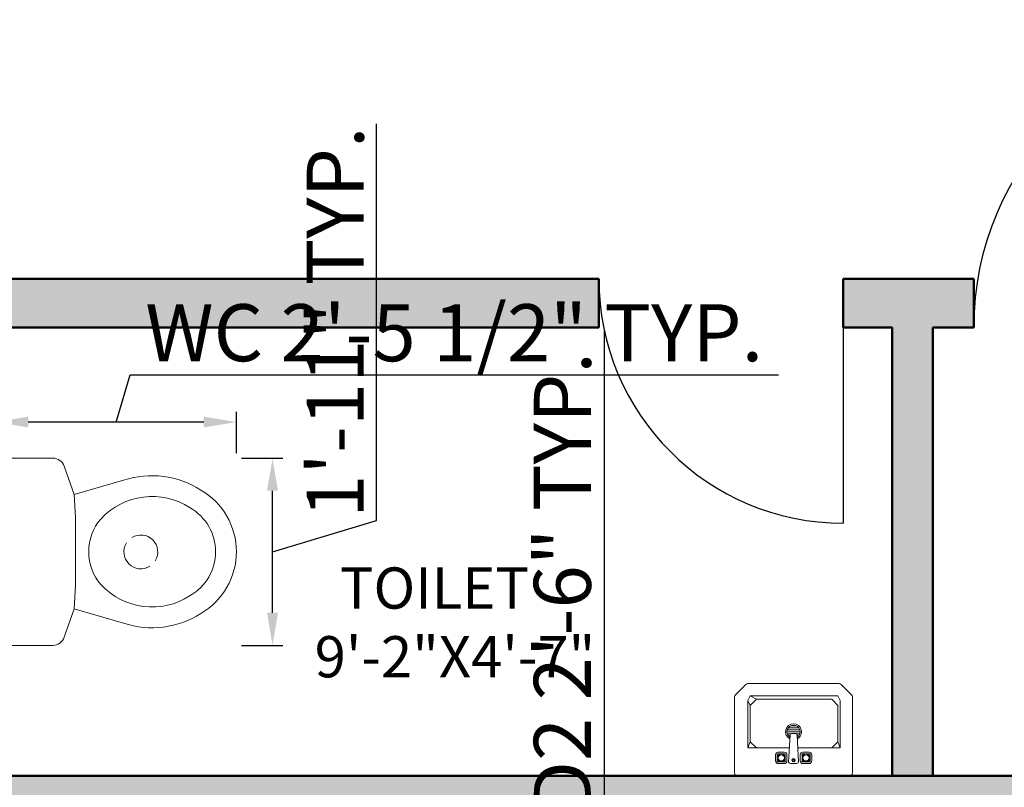
# Model space of a CAD drawing. Units: inches. Extents: x -7 to 1228, y -146 to 1091.
# Tile 51 of 88: x 72 to 193, y 786 to 880. Entities that reach past the tile are written whole.
import ezdxf

# ---------------------------------------------------------------- set-up
doc = ezdxf.new("R2010")
doc.units = ezdxf.units.IN
for name, color, linetype, lineweight in [('A-ANNO-DIMS', 2, 'Continuous', 18), ('A-AREA-IDEN', 7, 'Continuous', 18), ('A-DOOR', 4, 'Continuous', 25), ('A-FLOR-FIXT', 8, 'Continuous', 18), ('A-FURN', 8, 'Continuous', 18), ('A-WALL', 7, 'Continuous', 50), ('A-WALL-PATT', 251, 'Continuous', 13)]:
    doc.layers.add(name, color=color, linetype=linetype, lineweight=lineweight)
doc.styles.get("Standard").update_dxf_attribs({"font": 'arial.ttf'})
doc.dimstyles.new('ISO-25', dxfattribs={"dimtxt": 7, "dimasz": 4, "dimexe": 1.25, "dimexo": 0.625, "dimtad": 1, "dimdec": 1, "dimlunit": 3, "dimtxsty": 'Standard', "dimcen": 2.5, "dimadec": 0, "dimazin": 0, "dimtfac": 1, "dimtdec": 1, "dimtmove": 1, "dimatfit": 3, "dimfxl": 1, "dimarcsym": 0})

# ---------------------------------------------------------------- blocks, each defined once
blk = doc.blocks.new('A$C7B5C7CD4')
at = {"ltscale": 20}
for p, q in [((0, 0.614), (0, 0.4765)), ((0.243, 0.625), (0.011, 0.625)), ((0.243, 0.625), (0.475, 0.625)), ((0.486, 0.614), (0.486, 0.4765)), ((0.0212, 0.4467), (0.0946, 0.4214)), ((0.4648, 0.4467), (0.3914, 0.4214)), ((0.0946, 0.4214), (0.0576, 0.293)), ((0.0946, 0.4214), (0.1544, 0.4173)), ((0.3316, 0.4173), (0.1544, 0.4173)), ((0.3914, 0.4214), (0.3316, 0.4173)), ((0.3914, 0.4214), (0.4284, 0.293))]:
    blk.add_line(p, q, dxfattribs=at)
for centre, radius, start, end in [((0.011, 0.614), 0.011, 90, 180), ((0.475, 0.614), 0.011, 0, 90), ((0.0315, 0.4765), 0.0315, 180, 251), ((0.4545, 0.4765), 0.0315, 289, 0), ((0.24, 0.2602), 0.123, 88.6158, 131.7414), ((0.246, 0.2602), 0.123, 48.2586, 91.3842), ((0.2796, 0.219), 0.18, 132.4207, 213.289), ((0.2064, 0.219), 0.18, 326.711, 47.5793), ((0.2796, 0.219), 0.234, 161.5846, 212.8753), ((0.2064, 0.219), 0.234, 327.1247, 18.4154), ((0.243, 0.185), 0.131, 209.6292, 270), ((0.243, 0.185), 0.131, 270, 330.3708), ((0.243, 0.185), 0.185, 210.1745, 270), ((0.243, 0.185), 0.185, 270, 329.8255)]:
    blk.add_arc(centre, radius, start, end, dxfattribs=at)
for start, end in [(58.1785, 211.8215), (238.1785, 31.8215)]:
    blk.add_arc((0.2426, 0.2481), 0.0439, start, end)
blk = doc.blocks.new('A$C4CB854FF')
for p, q in [((0, 0.3675), (0, 0.0552)), ((0.4725, 0.38), (0.0125, 0.38)), ((0.485, 0.0552), (0.485, 0.3675)), ((0.1787, 0.329), (0.2034, 0.329)), ((0.2337, 0.329), (0.2502, 0.329)), ((0.3052, 0.329), (0.2804, 0.329)), ((0.1677, 0.2932), (0.1677, 0.318)), ((0.1745, 0.2919), (0.1745, 0.3194)), ((0.1773, 0.3221), (0.2048, 0.3221)), ((0.2048, 0.2891), (0.1773, 0.2891)), ((0.2075, 0.3194), (0.2075, 0.2919)), ((0.2144, 0.318), (0.2144, 0.2932)), ((0.2279, 0.2104), (0.2213, 0.3235)), ((0.2625, 0.3235), (0.256, 0.2104)), ((0.2694, 0.318), (0.2694, 0.2932)), ((0.2763, 0.3194), (0.2763, 0.2919)), ((0.3065, 0.3221), (0.279, 0.3221)), ((0.279, 0.2891), (0.3065, 0.2891)), ((0.3093, 0.2919), (0.3093, 0.3194)), ((0.3162, 0.2932), (0.3162, 0.318)), ((0.05, 0.265), (0.2247, 0.265)), ((0.06, 0.24), (0.05, 0.265)), ((0.05, 0.07), (0.05, 0.265)), ((0.085, 0.265), (0.06, 0.24)), ((0.2034, 0.2822), (0.1787, 0.2822)), ((0.2591, 0.265), (0.43, 0.265)), ((0.2804, 0.2822), (0.3052, 0.2822)), ((0.395, 0.265), (0.42, 0.24)), ((0.42, 0.24), (0.43, 0.265)), ((0.43, 0.07), (0.43, 0.265)), ((0.06, 0.24), (0.06, 0.09)), ((0.2297, 0.2066), (0.2165, 0.2066)), ((0.2272, 0.2149), (0.2208, 0.2149)), ((0.2505, 0.2052), (0.2334, 0.2052)), ((0.2681, 0.2066), (0.2541, 0.2066)), ((0.2638, 0.2149), (0.2566, 0.2149)), ((0.42, 0.24), (0.42, 0.09)), ((0.2152, 0.1984), (0.2694, 0.1984)), ((0.2681, 0.1901), (0.2165, 0.1901)), ((0.2638, 0.1819), (0.2208, 0.1819)), ((0.2533, 0.1736), (0.2313, 0.1736)), ((0.06, 0.09), (0.085, 0.065)), ((0.42, 0.09), (0.395, 0.065)), ((0.42, 0.09), (0.43, 0.07)), ((0.0037, 0.0463), (0.0463, 0.0037)), ((0.05, 0.07), (0.06, 0.05)), ((0.42, 0.05), (0.06, 0.05)), ((0.085, 0.065), (0.395, 0.065)), ((0.395, 0.065), (0.42, 0.05)), ((0.43, 0.07), (0.42, 0.05)), ((0.4387, 0.0037), (0.4813, 0.0463)), ((0.0552, 0), (0.4298, 0))]:
    blk.add_line(p, q)
for centre, radius in [((0.191, 0.3056), 0.0165), ((0.191, 0.3056), 0.0127), ((0.2419, 0.3152), 0.00688), ((0.2419, 0.3152), 0.00344), ((0.2928, 0.3056), 0.0165), ((0.2928, 0.3056), 0.0127)]:
    blk.add_circle(centre, radius)
for centre, radius, start, end in [((0.0125, 0.3675), 0.0125, 90, 180), ((0.4725, 0.3675), 0.0125, 0, 90), ((0.1787, 0.318), 0.011, 90, 180), ((0.2034, 0.318), 0.011, 0, 90), ((0.2329, 0.314), 0.015, 87.1975, 140.7274), ((0.2509, 0.314), 0.015, 39.2726, 92.8025), ((0.2804, 0.318), 0.011, 90, 180), ((0.3052, 0.318), 0.011, 0, 90), ((0.1787, 0.2932), 0.011, 180, 270), ((0.1773, 0.3194), 0.00275, 90, 180), ((0.1773, 0.2919), 0.00275, 180, 270), ((0.2034, 0.2932), 0.011, 270, 0), ((0.2048, 0.3194), 0.00275, 360, 90), ((0.2048, 0.2919), 0.00275, 270, 0), ((0.2804, 0.2932), 0.011, 180, 270), ((0.279, 0.3194), 0.00275, 90, 180), ((0.279, 0.2919), 0.00275, 180, 270), ((0.3052, 0.2932), 0.011, 270, 360), ((0.3065, 0.3194), 0.00275, 360, 90), ((0.3065, 0.2919), 0.00275, 270, 0), ((0.2423, 0.1984), 0.033, 118.6883, 62.8686), ((0.2423, 0.1984), 0.0271, 124.7758, 57.2247), ((0.2334, 0.2107), 0.0055, 183.3274, 270), ((0.2505, 0.2107), 0.0055, 270, 356.6726), ((0.0125, 0.0552), 0.0125, 180, 225), ((0.4725, 0.0552), 0.0125, 315, 0), ((0.0552, 0.0125), 0.0125, 225, 270), ((0.4298, 0.0125), 0.0125, 270, 315)]:
    blk.add_arc(centre, radius, start, end)
blk = doc.blocks.new('DOOR-750')
blk.add_line((30, 30), (30, 0))
blk.add_arc((30, 30), 30, 180, 270)
blk = doc.blocks.new('DOOR-900')
blk.add_line((36, 0), (36, 36))
blk.add_arc((36, 0), 36, 90, 180)
blk = doc.blocks.new('*D28')
at = {"layer": 'A-ANNO-DIMS', "color": 0, "lineweight": -2, "transparency": 16777216}
for p, q in [((83.77, 830.42), (85.51, 836.22)), ((85.51, 836.22), (165.04, 836.22)), ((69, 826.61), (69, 831.67)), ((98.54, 826.61), (98.54, 831.67)), ((94.54, 830.42), (73, 830.42))]:
    blk.add_line(p, q, dxfattribs=at)
at = {"layer": 'A-ANNO-DIMS', "color": 0, "transparency": 16777216}
for points in [[(73, 831.08), (73, 829.75), (69, 830.42)], [(94.54, 831.08), (94.54, 829.75), (98.54, 830.42)]]:
    blk.add_solid(points, dxfattribs=at)
at = {"layer": 'Defpoints', "color": 0, "transparency": 16777216}
for p in [(69, 830.42), (69, 825.98), (98.54, 825.98)]:
    blk.add_point(p, dxfattribs=at)
at = {"layer": 'A-ANNO-DIMS', "color": 0, "transparency": 16777216, "insert": (125.27, 840.47), "char_height": 7, "attachment_point": 5}
blk.add_mtext('WC 2\'-5 1/2" TYP.', dxfattribs=at)
blk = doc.blocks.new('*D29')
at = {"layer": 'A-ANNO-DIMS', "color": 0, "lineweight": -2, "transparency": 16777216}
for p, q in [((115.71, 818.32), (115.71, 867.02)), ((99.16, 825.98), (104.22, 825.98)), ((102.97, 807.02), (102.97, 821.98)), ((102.97, 814.5), (115.71, 818.32)), ((99.16, 803.02), (104.22, 803.02))]:
    blk.add_line(p, q, dxfattribs=at)
at = {"layer": 'A-ANNO-DIMS', "color": 0, "transparency": 16777216}
for points in [[(102.3, 821.98), (103.64, 821.98), (102.97, 825.98)], [(102.3, 807.02), (103.64, 807.02), (102.97, 803.02)]]:
    blk.add_solid(points, dxfattribs=at)
at = {"layer": 'Defpoints', "color": 0, "transparency": 16777216}
for p in [(98.54, 825.98), (102.97, 825.98), (98.54, 803.02)]:
    blk.add_point(p, dxfattribs=at)
at = {"layer": 'A-ANNO-DIMS', "color": 0, "transparency": 16777216, "insert": (111.57, 842.67), "char_height": 7, "attachment_point": 5, "rotation": 90}
blk.add_mtext('1\'-11" TYP.', dxfattribs=at)
blk = doc.blocks.new('*D46')
at = {"layer": 'A-ANNO-DIMS', "color": 0, "lineweight": -2, "transparency": 16777216}
for p, q in [((143.69, 750.74), (143.69, 841.58)), ((153.38, 764), (148.25, 764)), ((149.5, 760), (149.5, 738)), ((149.5, 749), (143.69, 750.74)), ((153.38, 734), (148.25, 734))]:
    blk.add_line(p, q, dxfattribs=at)
at = {"layer": 'A-ANNO-DIMS', "color": 0, "transparency": 16777216}
for points in [[(148.83, 760), (150.17, 760), (149.5, 764)], [(148.83, 738), (150.17, 738), (149.5, 734)]]:
    blk.add_solid(points, dxfattribs=at)
at = {"layer": 'Defpoints', "color": 0, "transparency": 16777216}
for p in [(154, 764), (149.5, 734), (154, 734)]:
    blk.add_point(p, dxfattribs=at)
at = {"layer": 'A-ANNO-DIMS', "color": 0, "transparency": 16777216, "insert": (139.44, 796.16), "char_height": 7, "attachment_point": 5, "rotation": 90}
blk.add_mtext('DOOR D2 2\'-6" TYP.', dxfattribs=at)

msp = doc.modelspace()

# ---------------------------------------------------------------- hatches: boundary and pattern name
at = {"layer": 'A-WALL-PATT'}
h = msp.add_hatch(color=256, dxfattribs=at)
h.dxf.hatch_style = 1
h.paths.add_polyline_path([(69, 568), (60, 568), (60, 493), (63.29, 493), (69, 493)])
h.paths.add_polyline_path([(69, 662.41), (60, 662.41), (60, 586), (69, 586)], flags=17)
h.paths.add_polyline_path([(69, 723), (184, 723), (184, 734), (179, 734), (179, 728), (69, 728), (69, 741.62), (60, 741.62), (60, 698.41), (69, 698.41)], flags=17)
h.paths.add_polyline_path([(69, 782), (231, 782), (231, 728), (231, 723), (231, 586), (236, 586), (236, 787), (69, 787), (69, 800.13), (60, 800.13), (60, 765.62), (69, 765.62)])
h.paths.add_polyline_path([(184, 842), (189, 842), (189, 848), (173, 848), (173, 842), (179, 842), (179, 787), (184, 787)])
h.paths.add_polyline_path([(118.22, 69), (69, 69), (69, 60), (118.22, 60)])
h.paths.add_polyline_path([(227, 69), (154.22, 69), (154.22, 60), (227, 60)])
h.paths.add_polyline_path([(236, 60), (232.71, 60), (227, 60), (227, 36), (236, 36)])
h.paths.add_polyline_path([(389, 60), (380, 60), (380, 36), (389, 36)])
h.paths.add_polyline_path([(384, 181), (380, 181), (380, 115), (380, 78), (384, 78)])
h.paths.add_polyline_path([(380, 115), (334.55, 115), (334.55, 109), (380, 109)])
h.paths.add_polyline_path([(274.55, 115), (236, 115), (236, 201), (232.71, 201), (231, 201), (231, 78), (236, 78), (236, 109), (274.55, 109)])
h.paths.add_polyline_path([(69, 123), (60, 123), (60, 78), (69, 78)])
h.paths.add_polyline_path([(69, 201), (60, 201), (60, 159), (69, 159)])
h.paths.add_polyline_path([(143, 219), (69, 219), (69, 213), (143, 213)], flags=17)
h.paths.add_polyline_path([(189, 219), (184, 219), (184, 274), (231, 274), (231, 219), (236, 219), (236, 279), (184, 279), (184, 297), (179, 297), (179, 279), (69, 279), (69, 290.91), (60, 290.91), (60, 262.18), (69, 262.18), (69, 274), (179, 274), (179, 219), (173, 219), (173, 213), (189, 213)])
h.paths.add_polyline_path([(69, 238.18), (60, 238.18), (60, 219), (69, 219)], flags=17)
h.paths.add_polyline_path([(69, 333), (60, 333), (60, 314.91), (69, 314.91), (69, 316.96)])
h.paths.add_polyline_path([(190, 338), (184, 338), (69, 338), (69, 333), (179, 333), (179, 327), (184, 327), (184, 333.02), (190, 333.05)])
h.paths.add_polyline_path([(69, 386.81), (60, 386.81), (60, 351), (69, 351)])
h.paths.add_polyline_path([(69, 475), (60, 475), (60, 422.81), (69, 422.81)])
h.paths.add_polyline_path([(236, 475), (231, 475), (231, 351.24), (236, 351.24)])
h.paths.add_polyline_path([(384, 475), (380, 475), (380, 362), (384, 362)])
h.paths.add_polyline_path([(547, 307), (439, 307), (439, 356), (445, 356), (445, 362), (433, 362), (433, 307), (380, 307), (380, 244), (380, 241), (384, 241), (384, 301), (433, 301), (433, 277), (439, 277), (439, 301), (547, 301)])
h.paths.add_polyline_path([(547, 241), (439, 241), (439, 247), (433, 247), (433, 235), (547, 235)])
h.paths.add_polyline_path([(450, 69), (440.29, 69), (424.89, 69), (389, 69), (389, 60), (450, 60)])
h.paths.add_polyline_path([(547, 69), (486, 69), (486, 60), (547, 60)])
h.paths.add_polyline_path([(556, 148.27), (547, 148.27), (547, 78), (556, 78)])
h.paths.add_polyline_path([(556, 223), (547, 223), (547, 195), (547, 184.27), (556, 184.27)])
h.paths.add_polyline_path([(556, 311.19), (547, 311.19), (547, 273.08), (556, 273.08)])
h.paths.add_polyline_path([(556, 344), (552.71, 344), (547, 344), (547, 335.19), (556, 335.19)])
h.paths.add_polyline_path([(556, 249.08), (547, 249.08), (547, 241), (556, 241)])
h.paths.add_polyline_path([(547, 362), (475, 362), (475, 356), (547, 356)], flags=0)
h.paths.add_polyline_path([(556, 399.62), (547, 399.62), (547, 362), (556, 362)])
h.paths.add_polyline_path([(556, 475), (547, 475), (547, 435.62), (556, 435.62)])
h.paths.add_polyline_path([(547, 493), (389, 493), (389, 487), (547, 487)])
h.paths.add_polyline_path([(380, 493), (278, 493), (278, 487), (380, 487)])
h.paths.add_polyline_path([(227, 493), (69, 493), (69, 487), (227, 487)])
h.paths.add_polyline_path([(643, 122.44), (634, 122.44), (634, 78), (643, 78)])
h.paths.add_polyline_path([(702.5, 69), (692.79, 69), (677.39, 69), (643, 69), (643, 60), (702.5, 60)])
h.paths.add_polyline_path([(798, 69), (738.5, 69), (738.5, 60), (798, 60)])
h.paths.add_polyline_path([(807, 60), (803.71, 60), (798, 60), (798, 36), (807, 36)])
h.paths.add_polyline_path([(807, 109), (846.75, 109), (846.75, 115), (807, 115), (807, 159), (802, 159), (802, 78), (807, 78)])
h.paths.add_polyline_path([(807, 201), (802, 201), (802, 195), (807, 195)])
h.paths.add_polyline_path([(643, 201), (634, 201), (634, 158.44), (643, 158.44)])
h.paths.add_polyline_path([(756, 225), (751, 225), (751, 219), (643, 219), (643, 213), (756, 213)])
h.paths.add_polyline_path([(643, 240.85), (634, 240.85), (634, 219), (643, 219)])
h.paths.add_polyline_path([(643, 274), (643, 288.63), (634, 288.63), (634, 264.85), (643, 264.85)])
h.paths.add_polyline_path([(802, 279), (756, 279), (756, 297), (751, 297), (751, 279), (643, 279), (643, 274), (751, 274), (751, 255), (756, 255), (756, 274), (802, 274)])
h.paths.add_polyline_path([(807, 333), (803.71, 333), (802, 333), (802, 279), (802, 274), (802, 219), (807, 219)])
h.paths.add_polyline_path([(956, 182), (951, 182), (951, 115), (906.75, 115), (906.75, 109), (951, 109), (951, 78), (956, 78)])
h.paths.add_polyline_path([(960, 60), (951, 60), (951, 36), (960, 36)])
h.paths.add_polyline_path([(1021, 69), (1005.78, 69), (960, 69), (960, 60), (1021, 60)])
h.paths.add_polyline_path([(956, 224), (951, 224), (951, 218), (956, 218)])
h.paths.add_polyline_path([(956, 302), (1004, 302), (1004, 278), (1010, 278), (1010, 302), (1118, 302), (1118, 290.81), (1127, 290.81), (1127, 326.97), (1118, 326.97), (1118, 320.97), (1118, 307), (1010, 307), (1010, 356), (1016, 356), (1016, 362), (1004, 362), (1004, 307), (951, 307), (951, 244), (951, 242), (954.29, 242), (956, 242)])
h.paths.add_polyline_path([(643, 333), (634, 333), (634, 312.63), (643, 312.63), (643, 316.96)])
h.paths.add_polyline_path([(756, 338), (643, 338), (643, 333), (751, 333), (751, 327), (756, 327)])
h.paths.add_polyline_path([(643, 388), (634, 388), (634, 351), (643, 351)])
h.paths.add_polyline_path([(807, 357), (802, 357), (802, 351), (807, 351)])
h.paths.add_polyline_path([(807, 475), (802, 475), (802, 393), (807, 393)])
h.paths.add_polyline_path([(643, 475), (634, 475), (634, 424), (643, 424)])
h.paths.add_polyline_path([(798, 493), (643, 493), (643, 487), (798, 487)])
h.paths.add_polyline_path([(634, 493), (556, 493), (556, 487), (634, 487)])
h.paths.add_polyline_path([(813, 493), (807, 493), (807, 487), (813, 487)])
h.paths.add_polyline_path([(951, 493), (849, 493), (849, 487), (951, 487)])
h.paths.add_polyline_path([(956, 484), (951, 484), (951, 374), (956, 374)])
h.paths.add_polyline_path([(1109, 493), (969, 493), (969, 487), (1109, 487)])
h.paths.add_polyline_path([(1127, 484), (1118, 484), (1118, 450.64), (1127, 450.64)])
h.paths.add_polyline_path([(1127, 414.64), (1118, 414.64), (1118, 365), (1127, 365)])
h.paths.add_polyline_path([(1109, 362), (1046, 362), (1046, 356), (1109, 356)], flags=17)
h.paths.add_polyline_path([(1127, 356), (1123.45, 356), (1118, 356), (1118, 350.97), (1127, 350.97)], flags=0)
h.paths.add_polyline_path([(1127, 266.81), (1118, 266.81), (1118, 262.36), (1118, 242), (1127, 242)], flags=17)
h.paths.add_polyline_path([(1118, 242), (1010, 242), (1010, 248), (1004, 248), (1004, 237), (1118, 237)])
h.paths.add_polyline_path([(1127, 224), (1118, 224), (1118, 170), (1127, 170)])
h.paths.add_polyline_path([(1127, 134), (1118, 134), (1118, 78), (1127, 78)])
h.paths.add_polyline_path([(1118, 69), (1057, 69), (1057, 60), (1118, 60)])
h.paths.add_polyline_path([(227, 571.55), (227, 574), (69, 574), (69, 568), (227, 568)])
h.paths.add_polyline_path([(380, 571.55), (380, 574), (278, 574), (278, 568), (380, 568)])
h.paths.add_polyline_path([(242, 574), (236, 574), (236, 568), (242, 568)])
h.paths.add_polyline_path([(547, 571.55), (547, 574), (389, 574), (389, 568), (547, 568)])
h.paths.add_polyline_path([(384, 733), (380, 733), (380, 586), (384, 586)])
h.paths.add_polyline_path([(556, 646), (634, 646), (634, 655), (547, 655), (547, 586), (556, 586)])
h.paths.add_polyline_path([(634, 574), (556, 574), (556, 568), (634, 568)])
h.paths.add_polyline_path([(643, 655), (634, 655), (634, 586), (643, 586)])
h.paths.add_polyline_path([(798, 574), (643, 574), (643, 568), (798, 568)])
h.paths.add_polyline_path([(643, 663.85), (634, 663.85), (634, 655), (643, 655)])
h.paths.add_polyline_path([(556, 676.97), (547, 676.97), (547, 655), (556, 655)])
h.paths.add_polyline_path([(556, 733), (547, 733), (547, 712.97), (556, 712.97)])
h.paths.add_polyline_path([(643, 710), (634, 710), (634, 699.85), (643, 699.85)])
h.paths.add_polyline_path([(807, 668), (802, 668), (802, 586), (807, 586)])
h.paths.add_polyline_path([(951, 574), (849, 574), (849, 568), (951, 568)])
h.paths.add_polyline_path([(956, 691), (951, 691), (951, 577), (956, 577)])
h.paths.add_polyline_path([(1109, 574), (969, 574), (969, 568), (1109, 568)])
h.paths.add_polyline_path([(1127, 643.4), (1118, 643.4), (1118, 577), (1127, 577)])
h.paths.add_polyline_path([(1127, 568), (1123.45, 568), (1118, 568), (1118, 493), (1127, 493)])
h.paths.add_polyline_path([(1127, 733), (1118, 733), (1118, 679.4), (1127, 679.4)])
h.paths.add_polyline_path([(1127, 777.35), (1118, 777.35), (1118, 770.04), (1118, 751), (1127, 751)], flags=17)
h.paths.add_polyline_path([(1118, 751), (1010, 751), (1010, 757), (1004, 757), (1004, 745), (1118, 745)])
h.paths.add_polyline_path([(956, 811), (1004, 811), (1004, 787), (1010, 787), (1010, 811), (1017.87, 811), (1017.87, 811.63, -0.414214), (1018.25, 812), (1031.98, 812, -0.414214), (1032.35, 811.63), (1032.35, 811), (1118, 811), (1118, 801.35), (1127, 801.35), (1127, 834.69), (1118, 834.69), (1118, 830.24), (1118, 817), (1010, 817), (1010, 866), (1016, 866), (1016, 872), (1004, 872), (1004, 817), (956, 817), (956, 866), (951, 866), (951, 751), (954.29, 751), (956, 751)])
h.paths.add_polyline_path([(1118, 872), (1046, 872), (1046, 866), (1118, 866)], flags=17)
h.paths.add_polyline_path([(1127, 924.71), (1118, 924.71), (1118, 884), (1127, 884)])
h.paths.add_polyline_path([(1127, 866), (1123.71, 866), (1118, 866), (1118, 858.69), (1127, 858.69)], flags=17)
h.paths.add_polyline_path([(956, 983), (951, 983), (951, 952), (807, 952), (807, 983), (802, 983), (802, 902), (807, 902), (807, 946), (951, 946), (951, 884), (956, 884)])
h.paths.add_polyline_path([(807, 842), (802, 842), (802, 787), (756, 787), (756, 806), (751, 806), (751, 787), (643, 787), (643, 782), (751, 782), (751, 764), (756, 764), (756, 782), (802, 782), (802, 728), (807, 728)])
h.paths.add_polyline_path([(756, 848), (643, 848), (643, 842), (751, 842), (751, 836), (756, 836)])
h.paths.add_polyline_path([(756, 734), (751, 734), (751, 728), (643, 728), (643, 723), (756, 723)])
h.paths.add_polyline_path([(643, 749.79), (634, 749.79), (634, 728), (637.29, 728), (643, 728)])
h.paths.add_polyline_path([(643, 805.41), (634, 805.41), (634, 773.79), (643, 773.79)])
h.paths.add_polyline_path([(643, 896.66), (634, 896.66), (634, 860), (637.29, 860), (643, 860)])
h.paths.add_polyline_path([(643, 842), (634, 842), (634, 829.41), (643, 829.41)])
h.paths.add_polyline_path([(643, 983), (634, 983), (634, 932.66), (643, 932.66)])
h.paths.add_polyline_path([(1127, 983), (1118, 983), (1118, 960.71), (1127, 960.71)])
h.paths.add_polyline_path([(1118, 1001), (1077.53, 1001), (1077.53, 992), (1118, 992)])
h.paths.add_polyline_path([(1041.53, 1001), (960, 1001), (960, 992), (1041.53, 992)])
h.paths.add_polyline_path([(960, 1025), (951, 1025), (951, 1001), (954.29, 1001), (960, 1001)])
h.paths.add_polyline_path([(807, 1025), (798, 1025), (798, 1001), (807, 1001)])
h.paths.add_polyline_path([(798, 1001), (738.5, 1001), (738.5, 992), (798, 992)])
h.paths.add_polyline_path([(702.5, 1001), (643, 1001), (643, 992), (702.5, 992)])
h.paths.add_polyline_path([(547, 1001), (499.11, 1001), (499.11, 992), (547, 992)])
h.paths.add_polyline_path([(463.11, 1001), (389, 1001), (389, 992), (463.11, 992)])
h.paths.add_polyline_path([(389, 1025), (380, 1025), (380, 1022), (380, 1001), (383.29, 1001), (389, 1001)])
h.paths.add_polyline_path([(236, 1025), (227, 1025), (227, 1001), (236, 1001)])
h.paths.add_polyline_path([(236, 983), (231, 983), (231, 860), (236, 860)])
h.paths.add_polyline_path([(274.55, 952), (236, 952), (236, 946), (274.55, 946)])
h.paths.add_polyline_path([(380, 952), (334.55, 952), (334.55, 946), (380, 946)])
h.paths.add_polyline_path([(384, 983), (380, 983), (380, 884), (383.29, 884), (384, 884)])
h.paths.add_polyline_path([(227, 1001), (155.01, 1001), (155.01, 992), (162.87, 992), (227, 992)])
h.paths.add_polyline_path([(119.01, 1001), (69, 1001), (69, 992), (119.01, 992)])
h.paths.add_polyline_path([(69, 983), (60, 983), (60, 922.99), (69, 922.99)])
h.paths.add_polyline_path([(69, 886.99), (60, 886.99), (60, 860), (63.29, 860), (69, 860)])
h.paths.add_polyline_path([(143, 848), (69, 848), (69, 842), (143, 842)])

# ---------------------------------------------------------------- linework, layer by layer
at = {"layer": 'A-WALL'}
for p, q in [((143, 848), (69, 848)), ((143, 848), (143, 842)), ((189, 848), (173, 848)), ((173, 842), (173, 848)), ((189, 842), (189, 848)), ((143, 842), (69, 842)), ((179, 842), (173, 842)), ((179, 842), (179, 787)), ((189, 842), (184, 842)), ((184, 842), (184, 787)), ((236, 787), (69, 787))]:
    msp.add_line(p, q, dxfattribs=at)

# ---------------------------------------------------------------- block references
at = {"layer": 'A-DOOR'}
for name, p in [('DOOR-900', (189, 842)), ('DOOR-750', (143, 818))]:
    msp.add_blockref(name, p, dxfattribs=at)
at = {"layer": 'A-FLOR-FIXT', "xscale": 47.26153857112405, "yscale": 47.26153857112405, "zscale": 47.26153857112405, "rotation": 90}
msp.add_blockref('A$C7B5C7CD4', (98.54, 803.02), dxfattribs=at)
at = {"layer": 'A-FURN', "xscale": 29.84864686937646, "yscale": 29.84864686937646, "zscale": 29.84864686937646, "rotation": 180}
msp.add_blockref('A$C4CB854FF', (174.13, 798.34), dxfattribs=at)

# ---------------------------------------------------------------- texts
at = {"layer": 'A-AREA-IDEN', "insert": (108.14, 812.58), "char_height": 5.0568, "attachment_point": 1}
msp.add_mtext_dynamic_manual_height_columns('  TOILET\\P9\'-2"X4\'-7"', width=137.2821, gutter_width=25.28, heights=[0], dxfattribs=at)

# ---------------------------------------------------------------- dimensions: what is measured, and where the dimension line sits
at = {"layer": 'A-ANNO-DIMS'}
for base, p1, p2, angle, text, picture, middle in [((102.97, 825.98), (98.54, 803.02), (98.54, 825.98), 90, '<> TYP.', '*D29', (111.57, 818.95)), ((69, 830.42), (98.54, 825.98), (69, 825.98), 180, 'WC <> TYP.', '*D28', (86.14, 840.47)), ((149.5, 734), (154, 764), (154, 734), 270, 'DOOR D2 <> TYP.', '*D46', (139.44, 751.37))]:
    dim = msp.add_linear_dim(base=base, p1=p1, p2=p2, angle=angle, text=text, dimstyle='ISO-25', override={"dimdec": 1, "dimlfac": 1, "dimrnd": 0, "dimzin": 1, "dimdsep": 46, "dimlunit": 4, "dimfrac": 2}, dxfattribs=at)
    dim.commit()
    dim.dimension.update_dxf_attribs({"geometry": picture, "text_midpoint": middle})

doc.saveas('drawing.dxf')
